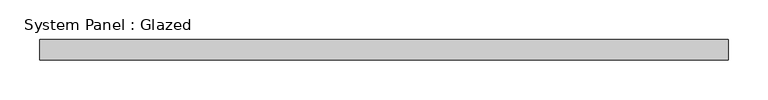
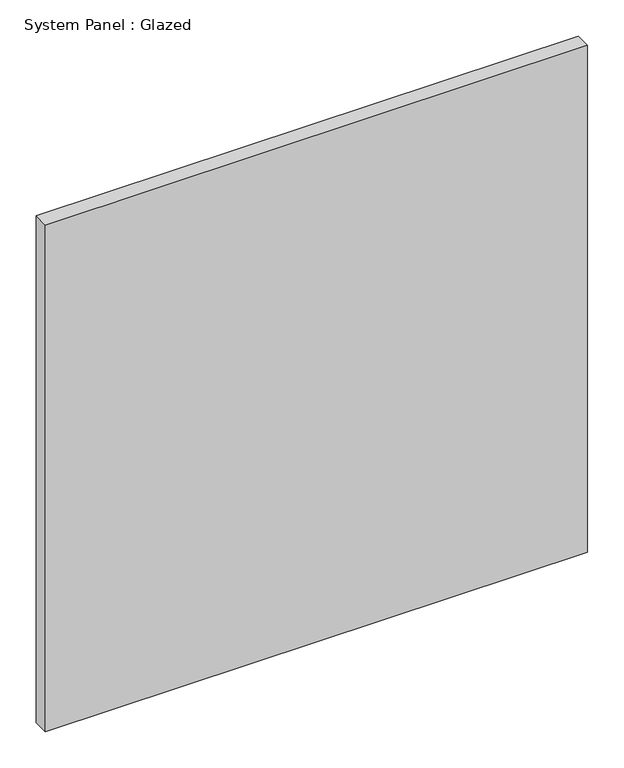
"""IFC4 building model written with IfcOpenShell, lengths in millimetres: plate geometry, System Panel : Glazed."""

from ifc_helpers import new_model, si_unit, origin, origin_with_axes, place, context, project, spatial, polyline, outline, extrude, source, transform, mapped, element, save


def system_panel_glazed_64bca335(model_context):
    return source(origin(), model_context, "Body", "SweptSolid", [
        extrude(outline(polyline([(431.8, 19.05), (-431.8, 19.05), (-431.8, 44.45), (431.8, 44.45), (431.8, 19.05)])), origin_with_axes(), (0.0, 0.0, 1.0), 853.0145651),
    ])


if __name__ == "__main__":
    model = new_model("IFC4")
    model_context = context("Model", 3, world=origin())
    ifc_project = project(units=[si_unit("LENGTHUNIT", "METRE", prefix="MILLI")], contexts=[model_context])
    site = spatial("IfcSite", under=ifc_project)
    building = spatial("IfcBuilding", under=site)
    placement = place(None, origin())
    system_panel_glazed_shape = system_panel_glazed_64bca335(model_context)
    element("IfcPlate", 1, ObjectType="System Panel : Glazed", at=placement, inside=building, context=model_context, shape_type="MappedRepresentation", body=[
        mapped(system_panel_glazed_shape, transform((0.0, 0.0, 0.0), x_axis=(1.0, 0.0, 0.0), y_axis=(0.0, 1.0, 0.0), z_axis=(0.0, 0.0, 1.0))),
    ])
    save(model, "model.ifc")

# Revit data of these elements
# Type "System Panel : Glazed"
#   Construction Type Id = "GSP4R"
#   Analytic Construction = "1/8 in Pilkington single glazing"
#   Visual Light Transmittance = 0.9
#   Solar Heat Gain Coefficient = 0.86
#   Heat Transfer Coefficient (U) = 1.18115 BTU/(h·ft²·°F)
#   Define Thermal Properties by = 1
# Element 1 (IfcPlate, "System Panel : Glazed")
#   Materials on its faces: "Glass"
# Materials
#   "Glass": class "Glass", colour RGB 0 128 192, transparency 0.75, Description = "Soda Lime Glass", Cost = 0
